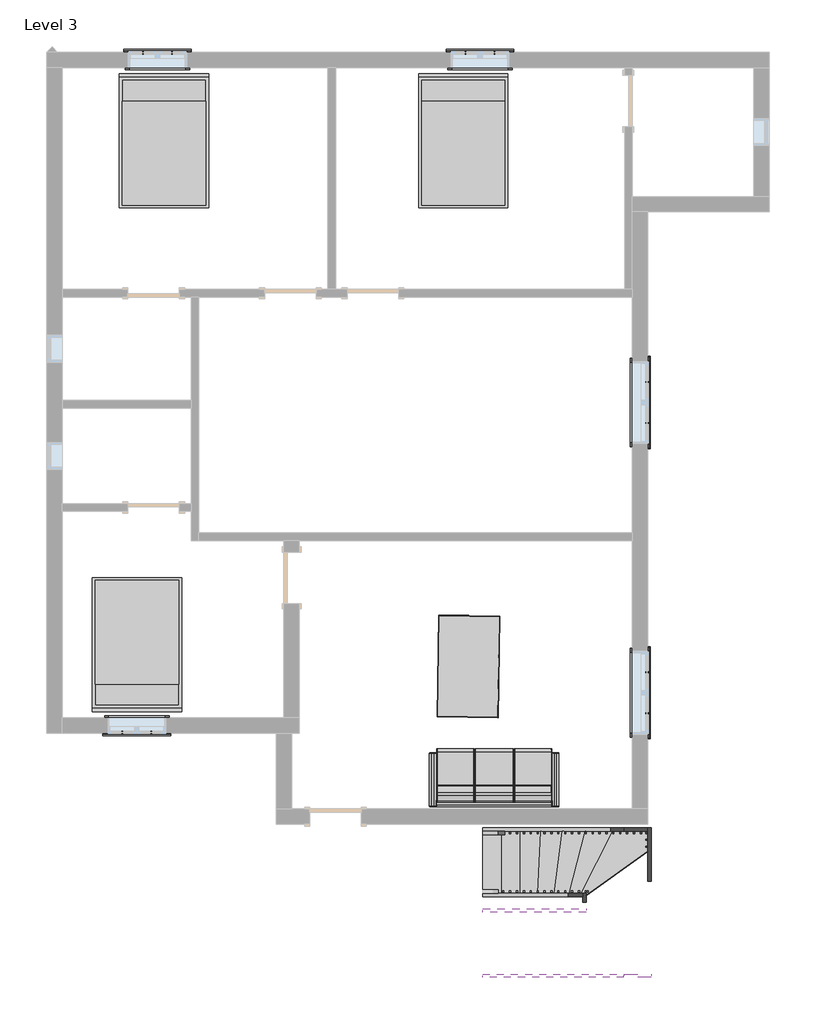
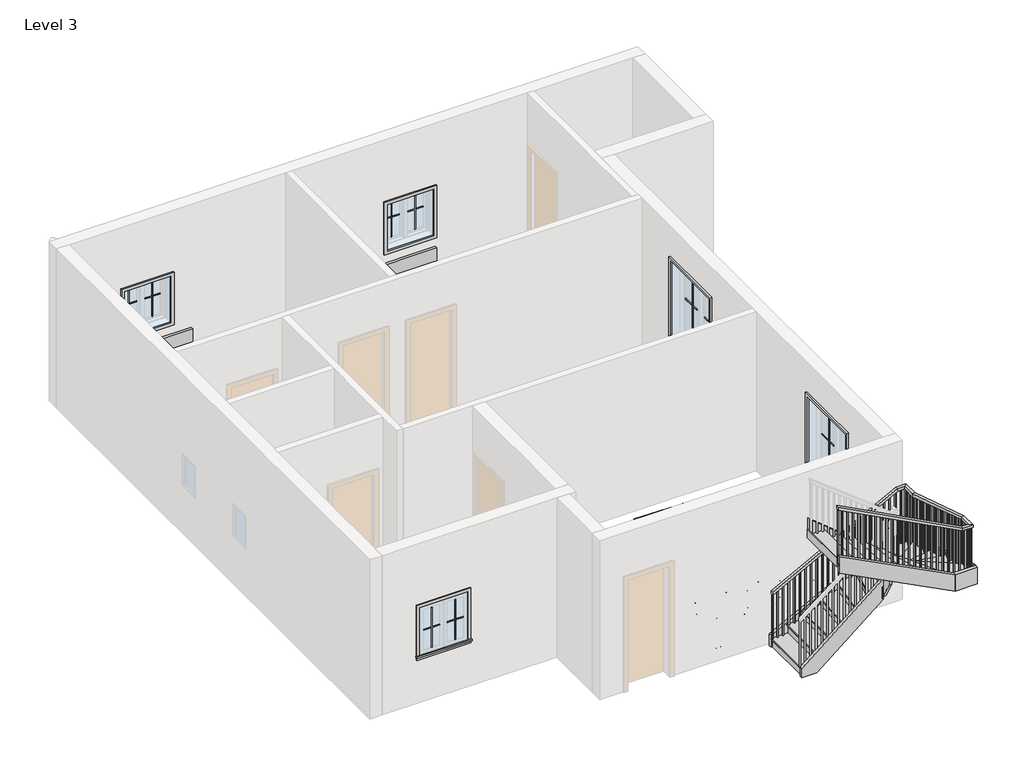
# One storey, part 2 of 2: 20 proxies, 8 members, 5 furniture elements, 1 railing, 1 stair flight.
"""IFC4 building model written with IfcOpenShell, lengths in millimetres."""

from ifc_helpers import new_model, si_unit, frame, origin, place, context, project, spatial, polyline, outline, extrude, faceted_brep, transform, mapped, element, save
from components import muntin_pattern_2x2_muntin_pattern_2x2_b3fe6957, muntin_pattern_2x2_muntin_pattern_2x2_3e0ecaf2, muntin_pattern_2x2_muntin_pattern_2x2_6dad3731, muntin_pattern_2x2_muntin_pattern_2x2_a30a3345, trim_window_exterior_flat_with_sill_41619996, trim_window_exterior_flat_with_sill_92b9b949, trim_window_interior_flat_picture_frame_51c85655, trim_window_interior_flat_picture_frame_3bb882cf, furniture_2fc85b74, furniture_29a9adb8, furniture_57072a26, bed_17739_bed_17739_15c61121, dining_table_14755_dining_table_14755_d89cb775, stair_flight_0756a42a

model = new_model("IFC4")

# Units and contexts
model_context = context("Model", 3, world=origin())
ifc_project = project(units=[si_unit("LENGTHUNIT", "METRE", prefix="MILLI")], contexts=[model_context])

# Site, building, storey
site = spatial("IfcSite", under=ifc_project)
building = spatial("IfcBuilding", under=site)
storey = spatial("IfcBuildingStorey", under=building, Name="Level 3", Elevation=3200.4)

# Proxies
placement = place(None, origin())
muntin_pattern_2x2_muntin_pattern_2x2_shape = muntin_pattern_2x2_muntin_pattern_2x2_b3fe6957(model_context)
element("IfcBuildingElementProxy", 1, Name="Muntin Pattern_2x2 : Muntin Pattern_2x2", ObjectType="Muntin Pattern_2x2 : Muntin Pattern_2x2", at=placement, inside=storey, context=model_context, shape_type="MappedRepresentation", body=[
    mapped(muntin_pattern_2x2_muntin_pattern_2x2_shape, transform((-4708.0540084, 8034.3685985, 4184.65), x_axis=(1.0, 0.0, 0.0), y_axis=(0.0, 1.0, 0.0), z_axis=(0.0, 0.0, 1.0))),
])
element("IfcBuildingElementProxy", 2, Name="Muntin Pattern_2x2 : Muntin Pattern_2x2", ObjectType="Muntin Pattern_2x2 : Muntin Pattern_2x2", at=placement, inside=storey, context=model_context, shape_type="MappedRepresentation", body=[
    mapped(muntin_pattern_2x2_muntin_pattern_2x2_shape, transform((54.4459916, 8034.3685985, 4184.65), x_axis=(1.0, 0.0, 0.0), y_axis=(0.0, 1.0, 0.0), z_axis=(0.0, 0.0, 1.0))),
])
element("IfcBuildingElementProxy", 3, Name="Muntin Pattern_2x2 : Muntin Pattern_2x2", ObjectType="Muntin Pattern_2x2 : Muntin Pattern_2x2", at=placement, inside=storey, context=model_context, shape_type="MappedRepresentation", body=[
    mapped(muntin_pattern_2x2_muntin_pattern_2x2_shape, transform((-4584.2290084, -2004.9814015, 4184.65), x_axis=(-1.0, 0.0, 0.0), y_axis=(0.0, -1.0, 0.0), z_axis=(0.0, 0.0, 1.0))),
])
muntin_pattern_2x2_muntin_pattern_2x2_2_shape = muntin_pattern_2x2_muntin_pattern_2x2_3e0ecaf2(model_context)
element("IfcBuildingElementProxy", 4, Name="Muntin Pattern_2x2 : Muntin Pattern_2x2", ObjectType="Muntin Pattern_2x2 : Muntin Pattern_2x2", at=placement, inside=storey, context=model_context, shape_type="MappedRepresentation", body=[
    mapped(muntin_pattern_2x2_muntin_pattern_2x2_2_shape, transform((-4279.4290084, 8034.3685985, 4184.65), x_axis=(-1.0, 0.0, 0.0), y_axis=(0.0, -1.0, 0.0), z_axis=(0.0, 0.0, 1.0))),
])
element("IfcBuildingElementProxy", 5, Name="Muntin Pattern_2x2 : Muntin Pattern_2x2", ObjectType="Muntin Pattern_2x2 : Muntin Pattern_2x2", at=placement, inside=storey, context=model_context, shape_type="MappedRepresentation", body=[
    mapped(muntin_pattern_2x2_muntin_pattern_2x2_2_shape, transform((483.0709916, 8034.3685985, 4184.65), x_axis=(-1.0, 0.0, 0.0), y_axis=(0.0, -1.0, 0.0), z_axis=(0.0, 0.0, 1.0))),
])
element("IfcBuildingElementProxy", 6, Name="Muntin Pattern_2x2 : Muntin Pattern_2x2", ObjectType="Muntin Pattern_2x2 : Muntin Pattern_2x2", at=placement, inside=storey, context=model_context, shape_type="MappedRepresentation", body=[
    mapped(muntin_pattern_2x2_muntin_pattern_2x2_2_shape, transform((-5012.8540084, -2004.9814015, 4184.65), x_axis=(1.0, 0.0, 0.0), y_axis=(0.0, 1.0, 0.0), z_axis=(0.0, 0.0, 1.0))),
])
muntin_pattern_2x2_muntin_pattern_2x2_3_shape = muntin_pattern_2x2_muntin_pattern_2x2_6dad3731(model_context)
element("IfcBuildingElementProxy", 7, Name="Muntin Pattern_2x2 : Muntin Pattern_2x2", ObjectType="Muntin Pattern_2x2 : Muntin Pattern_2x2", at=placement, inside=storey, context=model_context, shape_type="MappedRepresentation", body=[
    mapped(muntin_pattern_2x2_muntin_pattern_2x2_3_shape, transform((2735.7334916, -1114.3939015, 4184.65), x_axis=(0.0, -1.0, 0.0), y_axis=(1.0, 0.0, 0.0), z_axis=(0.0, 0.0, 1.0))),
])
element("IfcBuildingElementProxy", 8, Name="Muntin Pattern_2x2 : Muntin Pattern_2x2", ObjectType="Muntin Pattern_2x2 : Muntin Pattern_2x2", at=placement, inside=storey, context=model_context, shape_type="MappedRepresentation", body=[
    mapped(muntin_pattern_2x2_muntin_pattern_2x2_3_shape, transform((2735.7334916, 3171.8560985, 4184.65), x_axis=(0.0, -1.0, 0.0), y_axis=(1.0, 0.0, 0.0), z_axis=(0.0, 0.0, 1.0))),
])
muntin_pattern_2x2_muntin_pattern_2x2_4_shape = muntin_pattern_2x2_muntin_pattern_2x2_a30a3345(model_context)
element("IfcBuildingElementProxy", 9, Name="Muntin Pattern_2x2 : Muntin Pattern_2x2", ObjectType="Muntin Pattern_2x2 : Muntin Pattern_2x2", at=placement, inside=storey, context=model_context, shape_type="MappedRepresentation", body=[
    mapped(muntin_pattern_2x2_muntin_pattern_2x2_4_shape, transform((2735.7334916, -1720.8189015, 4184.65), x_axis=(0.0, 1.0, 0.0), y_axis=(-1.0, 0.0, 0.0), z_axis=(0.0, 0.0, 1.0))),
])
element("IfcBuildingElementProxy", 10, Name="Muntin Pattern_2x2 : Muntin Pattern_2x2", ObjectType="Muntin Pattern_2x2 : Muntin Pattern_2x2", at=placement, inside=storey, context=model_context, shape_type="MappedRepresentation", body=[
    mapped(muntin_pattern_2x2_muntin_pattern_2x2_4_shape, transform((2735.7334916, 2565.4310985, 4184.65), x_axis=(0.0, 1.0, 0.0), y_axis=(-1.0, 0.0, 0.0), z_axis=(0.0, 0.0, 1.0))),
])
trim_window_exterior_flat_with_sill_shape = trim_window_exterior_flat_with_sill_41619996(model_context)
element("IfcBuildingElementProxy", 11, Name="Trim-Window-Exterior-Flat : with Sill", ObjectType="Trim-Window-Exterior-Flat : with Sill", at=placement, inside=storey, context=model_context, shape_type="MappedRepresentation", body=[
    mapped(trim_window_exterior_flat_with_sill_shape, transform((-4493.7415084, 8043.8935985, 5029.2), x_axis=(-1.0, 0.0, 0.0), y_axis=(0.0, 0.0, 1.0), z_axis=(0.0, 1.0, 0.0))),
])
element("IfcBuildingElementProxy", 12, Name="Trim-Window-Exterior-Flat : with Sill", ObjectType="Trim-Window-Exterior-Flat : with Sill", at=placement, inside=storey, context=model_context, shape_type="MappedRepresentation", body=[
    mapped(trim_window_exterior_flat_with_sill_shape, transform((268.7584916, 8043.8935985, 5029.2), x_axis=(-1.0, 0.0, 0.0), y_axis=(0.0, 0.0, 1.0), z_axis=(0.0, 1.0, 0.0))),
])
element("IfcBuildingElementProxy", 13, Name="Trim-Window-Exterior-Flat : with Sill", ObjectType="Trim-Window-Exterior-Flat : with Sill", at=placement, inside=storey, context=model_context, shape_type="MappedRepresentation", body=[
    mapped(trim_window_exterior_flat_with_sill_shape, transform((-4798.5415084, -2014.5064015, 5029.2), x_axis=(1.0, 0.0, 0.0), y_axis=(0.0, 0.0, 1.0), z_axis=(0.0, -1.0, 0.0))),
])
trim_window_exterior_flat_with_sill_2_shape = trim_window_exterior_flat_with_sill_92b9b949(model_context)
element("IfcBuildingElementProxy", 14, Name="Trim-Window-Exterior-Flat : with Sill", ObjectType="Trim-Window-Exterior-Flat : with Sill", at=placement, inside=storey, context=model_context, shape_type="MappedRepresentation", body=[
    mapped(trim_window_exterior_flat_with_sill_2_shape, transform((2745.2584916, -1417.6064015, 5638.8), x_axis=(0.0, 1.0, 0.0), y_axis=(0.0, 0.0, 1.0), z_axis=(1.0, 0.0, 0.0))),
])
element("IfcBuildingElementProxy", 15, Name="Trim-Window-Exterior-Flat : with Sill", ObjectType="Trim-Window-Exterior-Flat : with Sill", at=placement, inside=storey, context=model_context, shape_type="MappedRepresentation", body=[
    mapped(trim_window_exterior_flat_with_sill_2_shape, transform((2745.2584916, 2868.6435985, 5638.8), x_axis=(0.0, 1.0, 0.0), y_axis=(0.0, 0.0, 1.0), z_axis=(1.0, 0.0, 0.0))),
])
trim_window_interior_flat_picture_frame_shape = trim_window_interior_flat_picture_frame_51c85655(model_context)
element("IfcBuildingElementProxy", 16, Name="Trim-Window-Interior-Flat : Picture Frame", ObjectType="Trim-Window-Interior-Flat : Picture Frame", at=placement, inside=storey, context=model_context, shape_type="MappedRepresentation", body=[
    mapped(trim_window_interior_flat_picture_frame_shape, transform((-4493.7415084, 7815.2935985, 5029.2), x_axis=(1.0, 0.0, 0.0), y_axis=(0.0, 0.0, 1.0), z_axis=(0.0, -1.0, 0.0))),
])
element("IfcBuildingElementProxy", 17, Name="Trim-Window-Interior-Flat : Picture Frame", ObjectType="Trim-Window-Interior-Flat : Picture Frame", at=placement, inside=storey, context=model_context, shape_type="MappedRepresentation", body=[
    mapped(trim_window_interior_flat_picture_frame_shape, transform((268.7584916, 7815.2935985, 5029.2), x_axis=(1.0, 0.0, 0.0), y_axis=(0.0, 0.0, 1.0), z_axis=(0.0, -1.0, 0.0))),
])
element("IfcBuildingElementProxy", 18, Name="Trim-Window-Interior-Flat : Picture Frame", ObjectType="Trim-Window-Interior-Flat : Picture Frame", at=placement, inside=storey, context=model_context, shape_type="MappedRepresentation", body=[
    mapped(trim_window_interior_flat_picture_frame_shape, transform((-4798.5415084, -1785.9064015, 5029.2), x_axis=(-1.0, 0.0, 0.0), y_axis=(0.0, 0.0, 1.0), z_axis=(0.0, 1.0, 0.0))),
])
trim_window_interior_flat_picture_frame_2_shape = trim_window_interior_flat_picture_frame_3bb882cf(model_context)
element("IfcBuildingElementProxy", 19, Name="Trim-Window-Interior-Flat : Picture Frame", ObjectType="Trim-Window-Interior-Flat : Picture Frame", at=placement, inside=storey, context=model_context, shape_type="MappedRepresentation", body=[
    mapped(trim_window_interior_flat_picture_frame_2_shape, transform((2516.6584916, -1417.6064015, 5638.8), x_axis=(0.0, -1.0, 0.0), y_axis=(0.0, 0.0, 1.0), z_axis=(-1.0, 0.0, 0.0))),
])
element("IfcBuildingElementProxy", 20, Name="Trim-Window-Interior-Flat : Picture Frame", ObjectType="Trim-Window-Interior-Flat : Picture Frame", at=placement, inside=storey, context=model_context, shape_type="MappedRepresentation", body=[
    mapped(trim_window_interior_flat_picture_frame_2_shape, transform((2516.6584916, 2868.6435985, 5638.8), x_axis=(0.0, -1.0, 0.0), y_axis=(0.0, 0.0, 1.0), z_axis=(-1.0, 0.0, 0.0))),
])

# Furniture
furniture_shape = furniture_2fc85b74(model_context)
furniture_2_shape = furniture_29a9adb8(model_context)
furniture_3_shape = furniture_57072a26(model_context)
element("IfcFurniture", 21, at=placement, inside=storey, context=model_context, shape_type="MappedRepresentation", body=[
    mapped(furniture_shape, transform((477.9947981, -2301.7922014, 3200.4), x_axis=(-1.0, 0.0, 0.0), y_axis=(0.0, -1.0, 0.0), z_axis=(0.0, 0.0, 1.0))),
    mapped(furniture_2_shape, transform((477.9947981, -2301.7922014, 3200.4), x_axis=(-1.0, 0.0, 0.0), y_axis=(0.0, -1.0, 0.0), z_axis=(0.0, 0.0, 1.0))),
    mapped(furniture_3_shape, transform((477.9947981, -2301.7922014, 3200.4), x_axis=(-1.0, 0.0, 0.0), y_axis=(0.0, -1.0, 0.0), z_axis=(0.0, 0.0, 1.0))),
])
bed_17739_bed_17739_shape = bed_17739_bed_17739_15c61121(model_context)
element("IfcFurniture", 22, ObjectType="Bed_17739 : Bed_17739", at=placement, inside=storey, context=model_context, shape_type="MappedRepresentation", body=[
    mapped(bed_17739_bed_17739_shape, transform((-4398.4915084, 6710.3935985, 3200.4), x_axis=(1.0, 0.0, 0.0), y_axis=(0.0, 1.0, 0.0), z_axis=(0.0, 0.0, 1.0))),
])
element("IfcFurniture", 23, ObjectType="Bed_17739 : Bed_17739", at=placement, inside=storey, context=model_context, shape_type="MappedRepresentation", body=[
    mapped(bed_17739_bed_17739_shape, transform((21.1084916, 6710.3935985, 3200.4), x_axis=(1.0, 0.0, 0.0), y_axis=(0.0, 1.0, 0.0), z_axis=(0.0, 0.0, 1.0))),
])
element("IfcFurniture", 24, ObjectType="Bed_17739 : Bed_17739", at=placement, inside=storey, context=model_context, shape_type="MappedRepresentation", body=[
    mapped(bed_17739_bed_17739_shape, transform((-4798.5415084, -681.0064015, 3200.4), x_axis=(-1.0, 0.0, 0.0), y_axis=(0.0, -1.0, 0.0), z_axis=(0.0, 0.0, 1.0))),
])
dining_table_14755_dining_table_14755_shape = dining_table_14755_dining_table_14755_d89cb775(model_context)
element("IfcFurniture", 25, ObjectType="Dining_table_14755 : Dining_table_14755", at=placement, inside=storey, context=model_context, shape_type="MappedRepresentation", body=[
    mapped(dining_table_14755_dining_table_14755_shape, transform((535.647979, -1785.9064015, 3200.4), x_axis=(0.016088397262737867, 0.9998705733611308, 0.0), y_axis=(-0.9998705733611308, 0.016088397262737867, 0.0), z_axis=(0.0, 0.0, 1.0))),
])

# Members
element("IfcMember", 26, ObjectType="Stringer - 2\" Width", at=placement, inside=storey, context=model_context, shape_type="SweptSolid", body=[
    extrude(outline(polyline([(3430.039954, 306.9570026), (3200.4, 306.9570026), (3200.4, 526.7193201), (4162.900629, 2394.3741942), (4505.7956453, 2394.3741942), (3430.039954, 306.9570026)])), frame((0.0, -3462.3064015, 0.0), z_axis=(0.0, 1.0, 0.0), x_axis=(0.0, 0.0, 1.0)), (0.0, 0.0, 1.0), 50.8),
])
element("IfcMember", 27, ObjectType="Stringer - 2\" Width", at=placement, inside=storey, context=model_context, shape_type="SweptSolid", body=[
    extrude(outline(polyline([(2394.3741942, -3462.3064015), (2394.3741942, -3411.5064015), (2749.0886944, -3411.5064015), (2749.0886944, -3462.3064015), (2394.3741942, -3462.3064015)])), frame((0.0, 0.0, 4162.900629), z_axis=(0.0, 0.0, 1.0), x_axis=(1.0, 0.0, 0.0)), (0.0, 0.0, 1.0), 342.8950162),
])
element("IfcMember", 28, ObjectType="Stringer - 2\" Width", at=placement, inside=storey, context=model_context, shape_type="SweptSolid", body=[
    extrude(outline(polyline([(-3411.5064015, 4489.4952212), (-3411.5064015, 4200.9956453), (-3581.0288845, 4200.9956453), (-5570.5064015, 4839.3682298), (-5570.5064015, 5170.3972697), (-5533.5262842, 5170.3972697), (-3411.5064015, 4489.4952212)])), frame((2749.0886944, 0.0, 0.0), z_axis=(1.0, 0.0, 0.0), x_axis=(0.0, 1.0, 0.0)), (0.0, 0.0, 1.0), 50.8),
])
element("IfcMember", 29, ObjectType="Stringer - 2\" Width", at=placement, inside=storey, context=model_context, shape_type="SweptSolid", body=[
    extrude(outline(polyline([(2799.8886944, -5570.5064015), (2799.8886944, -5621.3064015), (2394.3741942, -5621.3064015), (2394.3741942, -5570.5064015), (2799.8886944, -5570.5064015)])), frame((0.0, 0.0, 4850.2904473), z_axis=(0.0, 0.0, 1.0), x_axis=(1.0, 0.0, 0.0)), (0.0, 0.0, 1.0), 320.1068224),
])
element("IfcMember", 30, ObjectType="Stringer - 2\" Width", at=placement, inside=storey, context=model_context, shape_type="SweptSolid", body=[
    extrude(outline(polyline([(4850.2904473, 2394.3741942), (5170.3972697, 2394.3741942), (6246.1529609, 306.9570026), (5926.0461385, 306.9570026), (4850.2904473, 2394.3741942)])), frame((0.0, -5621.3064015, 0.0), z_axis=(0.0, 1.0, 0.0), x_axis=(0.0, 0.0, 1.0)), (0.0, 0.0, 1.0), 50.8),
])
element("IfcMember", 31, ObjectType="Stringer - 2\" Width", at=placement, inside=storey, context=model_context, shape_type="SweptSolid", body=[
    extrude(outline(polyline([(3376.5764461, 306.9570026), (3200.4, 306.9570026), (3200.4, 573.2186471), (4187.5410923, 1783.8886944), (4580.818648, 1783.8886944), (3376.5764461, 306.9570026)])), frame((0.0, -4427.5064015, 0.0), z_axis=(0.0, 1.0, 0.0), x_axis=(0.0, 0.0, 1.0)), (0.0, 0.0, 1.0), 50.8),
])
element("IfcMember", 32, ObjectType="Stringer - 2\" Width", at=placement, inside=storey, context=model_context, shape_type="SweptSolid", body=[
    extrude(outline(polyline([(-4376.7064015, 4773.6682978), (-4376.7064015, 4228.9617647), (-4410.9486188, 4228.9617647), (-4605.3064015, 4560.865107), (-4605.3064015, 5126.5409689), (-4583.3435189, 5126.5409689), (-4376.7064015, 4773.6682978)])), frame((1783.8886944, 0.0, 0.0), z_axis=(1.0, 0.0, 0.0), x_axis=(0.0, 1.0, 0.0)), (0.0, 0.0, 1.0), 50.8),
])
element("IfcMember", 33, ObjectType="Stringer - 2\" Width", at=placement, inside=storey, context=model_context, shape_type="SweptSolid", body=[
    extrude(outline(polyline([(4733.2634131, 1834.6886944), (5126.5409689, 1834.6886944), (6372.2038432, 306.9570026), (5978.9262875, 306.9570026), (4733.2634131, 1834.6886944)])), frame((0.0, -4656.1064015, 0.0), z_axis=(0.0, 1.0, 0.0), x_axis=(0.0, 0.0, 1.0)), (0.0, 0.0, 1.0), 50.8),
])

# Railing
element("IfcRailing", 34, ObjectType="Handrail - Rectangular", at=placement, inside=storey, context=model_context, shape_type="SolidModel", body=[
    faceted_brep([(306.9570026, -3462.3064015, 4284.1333333), (306.9570026, -3462.3064015, 4226.6742652), (306.9570026, -3513.1064015, 4226.6742652), (306.9570026, -3513.1064015, 4284.1333333), (2564.6820646, -3462.3064015, 5477.4239201), (2577.2811291, -3462.3064015, 5426.6239201), (2577.2811291, -3513.1064015, 5426.6239201), (2564.6820646, -3513.1064015, 5477.4239201), (2749.0886944, -3462.3064015, 5477.4239201), (2749.0886944, -3462.3064015, 5426.6239201), (2698.2886944, -3513.1064015, 5426.6239201), (2698.2886944, -3513.1064015, 5477.4239201), (2749.0886944, -3749.6182836, 5477.4239201), (2749.0886944, -3757.5688598, 5426.6239201), (2698.2886944, -3757.5688598, 5426.6239201), (2698.2886944, -3749.6182836, 5477.4239201), (2749.0886944, -5283.1945194, 5969.5094132), (2749.0886944, -5291.1450955, 5918.7094132), (2698.2886944, -5291.1450955, 5918.7094132), (2698.2886944, -5283.1945194, 5969.5094132), (2749.0886944, -5570.5064015, 5969.5094132), (2749.0886944, -5570.5064015, 5918.7094132), (2698.2886944, -5519.7064015, 5918.7094132), (2698.2886944, -5519.7064015, 5969.5094132), (2564.6820646, -5570.5064015, 5969.5094132), (2552.0830001, -5570.5064015, 5918.7094132), (2552.0830001, -5519.7064015, 5918.7094132), (2564.6820646, -5519.7064015, 5969.5094132), (306.9570026, -5570.5064015, 7162.8), (306.9570026, -5519.7064015, 7162.8), (306.9570026, -5519.7064015, 7105.3409318), (306.9570026, -5570.5064015, 7105.3409318)], [[[0, 1, 2, 3]], [[1, 0, 4, 5]], [[2, 1, 5, 6]], [[3, 2, 6, 7]], [[0, 3, 7, 4]], [[5, 4, 8, 9]], [[6, 5, 9, 10]], [[7, 6, 10, 11]], [[4, 7, 11, 8]], [[9, 8, 12, 13]], [[10, 9, 13, 14]], [[11, 10, 14, 15]], [[8, 11, 15, 12]], [[13, 12, 16, 17]], [[14, 13, 17, 18]], [[15, 14, 18, 19]], [[12, 15, 19, 16]], [[17, 16, 20, 21]], [[18, 17, 21, 22]], [[19, 18, 22, 23]], [[16, 19, 23, 20]], [[21, 20, 24, 25]], [[22, 21, 25, 26]], [[23, 22, 26, 27]], [[20, 23, 27, 24]], [[28, 29, 30, 31]], [[25, 24, 28, 31]], [[26, 25, 31, 30]], [[27, 26, 30, 29]], [[24, 27, 29, 28]]]),
    extrude(outline(polyline([(7068.1284102, 377.3636944), (6079.0666667, 377.3636944), (6079.0666667, 396.4136944), (7058.0597858, 396.4136944), (7068.1284102, 377.3636944)])), frame((0.0, -5554.6314015, 0.0), z_axis=(0.0, 1.0, 0.0), x_axis=(0.0, 0.0, 1.0)), (0.0, 0.0, 1.0), 19.05),
    extrude(outline(polyline([(7014.42908, 478.9636944), (6079.0666667, 478.9636944), (6079.0666667, 498.0136944), (7004.3604556, 498.0136944), (7014.42908, 478.9636944)])), frame((0.0, -5554.6314015, 0.0), z_axis=(0.0, 1.0, 0.0), x_axis=(0.0, 0.0, 1.0)), (0.0, 0.0, 1.0), 19.05),
    extrude(outline(polyline([(6960.7297498, 580.5636944), (5909.7333333, 580.5636944), (5909.7333333, 599.6136944), (6950.6611254, 599.6136944), (6960.7297498, 580.5636944)])), frame((0.0, -5554.6314015, 0.0), z_axis=(0.0, 1.0, 0.0), x_axis=(0.0, 0.0, 1.0)), (0.0, 0.0, 1.0), 19.05),
    extrude(outline(polyline([(6907.0304196, 682.1636944), (5909.7333333, 682.1636944), (5909.7333333, 701.2136944), (6896.9617952, 701.2136944), (6907.0304196, 682.1636944)])), frame((0.0, -5554.6314015, 0.0), z_axis=(0.0, 1.0, 0.0), x_axis=(0.0, 0.0, 1.0)), (0.0, 0.0, 1.0), 19.05),
    extrude(outline(polyline([(6853.3310894, 783.7636944), (5909.7333333, 783.7636944), (5909.7333333, 802.8136944), (6843.262465, 802.8136944), (6853.3310894, 783.7636944)])), frame((0.0, -5554.6314015, 0.0), z_axis=(0.0, 1.0, 0.0), x_axis=(0.0, 0.0, 1.0)), (0.0, 0.0, 1.0), 19.05),
    extrude(outline(polyline([(6799.6317592, 885.3636944), (5740.4, 885.3636944), (5740.4, 904.4136944), (6789.5631348, 904.4136944), (6799.6317592, 885.3636944)])), frame((0.0, -5554.6314015, 0.0), z_axis=(0.0, 1.0, 0.0), x_axis=(0.0, 0.0, 1.0)), (0.0, 0.0, 1.0), 19.05),
    extrude(outline(polyline([(6745.932429, 986.9636944), (5740.4, 986.9636944), (5740.4, 1006.0136944), (6735.8638046, 1006.0136944), (6745.932429, 986.9636944)])), frame((0.0, -5554.6314015, 0.0), z_axis=(0.0, 1.0, 0.0), x_axis=(0.0, 0.0, 1.0)), (0.0, 0.0, 1.0), 19.05),
    extrude(outline(polyline([(6692.2330988, 1088.5636944), (5740.4, 1088.5636944), (5740.4, 1107.6136944), (6682.1644744, 1107.6136944), (6692.2330988, 1088.5636944)])), frame((0.0, -5554.6314015, 0.0), z_axis=(0.0, 1.0, 0.0), x_axis=(0.0, 0.0, 1.0)), (0.0, 0.0, 1.0), 19.05),
    extrude(outline(polyline([(6638.5337686, 1190.1636944), (5571.0666667, 1190.1636944), (5571.0666667, 1209.2136944), (6628.4651442, 1209.2136944), (6638.5337686, 1190.1636944)])), frame((0.0, -5554.6314015, 0.0), z_axis=(0.0, 1.0, 0.0), x_axis=(0.0, 0.0, 1.0)), (0.0, 0.0, 1.0), 19.05),
    extrude(outline(polyline([(6584.8344384, 1291.7636944), (5571.0666667, 1291.7636944), (5571.0666667, 1310.8136944), (6574.765814, 1310.8136944), (6584.8344384, 1291.7636944)])), frame((0.0, -5554.6314015, 0.0), z_axis=(0.0, 1.0, 0.0), x_axis=(0.0, 0.0, 1.0)), (0.0, 0.0, 1.0), 19.05),
    extrude(outline(polyline([(6531.1351082, 1393.3636944), (5571.0666667, 1393.3636944), (5571.0666667, 1412.4136944), (6521.0664838, 1412.4136944), (6531.1351082, 1393.3636944)])), frame((0.0, -5554.6314015, 0.0), z_axis=(0.0, 1.0, 0.0), x_axis=(0.0, 0.0, 1.0)), (0.0, 0.0, 1.0), 19.05),
    extrude(outline(polyline([(6477.435778, 1494.9636944), (5401.7333333, 1494.9636944), (5401.7333333, 1514.0136944), (6467.3671536, 1514.0136944), (6477.435778, 1494.9636944)])), frame((0.0, -5554.6314015, 0.0), z_axis=(0.0, 1.0, 0.0), x_axis=(0.0, 0.0, 1.0)), (0.0, 0.0, 1.0), 19.05),
    extrude(outline(polyline([(6423.7364478, 1596.5636944), (5401.7333333, 1596.5636944), (5401.7333333, 1615.6136944), (6413.6678234, 1615.6136944), (6423.7364478, 1596.5636944)])), frame((0.0, -5554.6314015, 0.0), z_axis=(0.0, 1.0, 0.0), x_axis=(0.0, 0.0, 1.0)), (0.0, 0.0, 1.0), 19.05),
    extrude(outline(polyline([(6370.0371176, 1698.1636944), (5401.7333333, 1698.1636944), (5401.7333333, 1717.2136944), (6359.9684932, 1717.2136944), (6370.0371176, 1698.1636944)])), frame((0.0, -5554.6314015, 0.0), z_axis=(0.0, 1.0, 0.0), x_axis=(0.0, 0.0, 1.0)), (0.0, 0.0, 1.0), 19.05),
    extrude(outline(polyline([(6316.3377874, 1799.7636944), (5401.7333333, 1799.7636944), (5401.7333333, 1818.8136944), (6306.269163, 1818.8136944), (6316.3377874, 1799.7636944)])), frame((0.0, -5554.6314015, 0.0), z_axis=(0.0, 1.0, 0.0), x_axis=(0.0, 0.0, 1.0)), (0.0, 0.0, 1.0), 19.05),
    extrude(outline(polyline([(6262.6384572, 1901.3636944), (5232.4, 1901.3636944), (5232.4, 1920.4136944), (6252.5698328, 1920.4136944), (6262.6384572, 1901.3636944)])), frame((0.0, -5554.6314015, 0.0), z_axis=(0.0, 1.0, 0.0), x_axis=(0.0, 0.0, 1.0)), (0.0, 0.0, 1.0), 19.05),
    extrude(outline(polyline([(6208.939127, 2002.9636944), (5232.4, 2002.9636944), (5232.4, 2022.0136944), (6198.8705026, 2022.0136944), (6208.939127, 2002.9636944)])), frame((0.0, -5554.6314015, 0.0), z_axis=(0.0, 1.0, 0.0), x_axis=(0.0, 0.0, 1.0)), (0.0, 0.0, 1.0), 19.05),
    extrude(outline(polyline([(6155.2397968, 2104.5636944), (5232.4, 2104.5636944), (5232.4, 2123.6136944), (6145.1711724, 2123.6136944), (6155.2397968, 2104.5636944)])), frame((0.0, -5554.6314015, 0.0), z_axis=(0.0, 1.0, 0.0), x_axis=(0.0, 0.0, 1.0)), (0.0, 0.0, 1.0), 19.05),
    extrude(outline(polyline([(6101.5404666, 2206.1636944), (5232.4, 2206.1636944), (5232.4, 2225.2136944), (6091.4718422, 2225.2136944), (6101.5404666, 2206.1636944)])), frame((0.0, -5554.6314015, 0.0), z_axis=(0.0, 1.0, 0.0), x_axis=(0.0, 0.0, 1.0)), (0.0, 0.0, 1.0), 19.05),
    extrude(outline(polyline([(6047.8411364, 2307.7636944), (5063.0666667, 2307.7636944), (5063.0666667, 2326.8136944), (6037.772512, 2326.8136944), (6047.8411364, 2307.7636944)])), frame((0.0, -5554.6314015, 0.0), z_axis=(0.0, 1.0, 0.0), x_axis=(0.0, 0.0, 1.0)), (0.0, 0.0, 1.0), 19.05),
    extrude(outline(polyline([(5994.1418062, 2409.3636944), (5063.0666667, 2409.3636944), (5063.0666667, 2428.4136944), (5984.0731818, 2428.4136944), (5994.1418062, 2409.3636944)])), frame((0.0, -5554.6314015, 0.0), z_axis=(0.0, 1.0, 0.0), x_axis=(0.0, 0.0, 1.0)), (0.0, 0.0, 1.0), 19.05),
    extrude(outline(polyline([(5940.442476, 2510.9636944), (5063.0666667, 2510.9636944), (5063.0666667, 2530.0136944), (5930.3738516, 2530.0136944), (5940.442476, 2510.9636944)])), frame((0.0, -5554.6314015, 0.0), z_axis=(0.0, 1.0, 0.0), x_axis=(0.0, 0.0, 1.0)), (0.0, 0.0, 1.0), 19.05),
    extrude(outline(polyline([(2631.6136944, -5554.6314015), (2612.5636944, -5554.6314015), (2612.5636944, -5535.5814015), (2631.6136944, -5535.5814015), (2631.6136944, -5554.6314015)])), frame((0.0, 0.0, 5063.0666667), z_axis=(0.0, 0.0, 1.0), x_axis=(1.0, 0.0, 0.0)), (0.0, 0.0, 1.0), 855.6427466),
    extrude(outline(polyline([(2733.2136944, -5510.1814015), (2733.2136944, -5529.2314015), (2714.1636944, -5529.2314015), (2714.1636944, -5510.1814015), (2733.2136944, -5510.1814015)])), frame((0.0, 0.0, 5063.0666667), z_axis=(0.0, 0.0, 1.0), x_axis=(1.0, 0.0, 0.0)), (0.0, 0.0, 1.0), 855.6427466),
    extrude(outline(polyline([(2733.2136944, -5408.5814015), (2733.2136944, -5427.6314015), (2714.1636944, -5427.6314015), (2714.1636944, -5408.5814015), (2733.2136944, -5408.5814015)])), frame((0.0, 0.0, 5063.0666667), z_axis=(0.0, 0.0, 1.0), x_axis=(1.0, 0.0, 0.0)), (0.0, 0.0, 1.0), 855.6427466),
    extrude(outline(polyline([(2733.2136944, -5306.9814015), (2733.2136944, -5326.0314015), (2714.1636944, -5326.0314015), (2714.1636944, -5306.9814015), (2733.2136944, -5306.9814015)])), frame((0.0, 0.0, 5063.0666667), z_axis=(0.0, 0.0, 1.0), x_axis=(1.0, 0.0, 0.0)), (0.0, 0.0, 1.0), 855.6427466),
    extrude(outline(polyline([(-5205.3814015, 5891.1900316), (-5205.3814015, 4893.7333333), (-5224.4314015, 4893.7333333), (-5224.4314015, 5897.3026907), (-5205.3814015, 5891.1900316)])), frame((2714.1636944, 0.0, 0.0), z_axis=(1.0, 0.0, 0.0), x_axis=(0.0, 1.0, 0.0)), (0.0, 0.0, 1.0), 19.05),
    extrude(outline(polyline([(-5103.7814015, 5858.5891834), (-5103.7814015, 4893.7333333), (-5122.8314015, 4893.7333333), (-5122.8314015, 5864.7018425), (-5103.7814015, 5858.5891834)])), frame((2714.1636944, 0.0, 0.0), z_axis=(1.0, 0.0, 0.0), x_axis=(0.0, 1.0, 0.0)), (0.0, 0.0, 1.0), 19.05),
    extrude(outline(polyline([(-5002.1814015, 5825.9883352), (-5002.1814015, 4893.7333333), (-5021.2314015, 4893.7333333), (-5021.2314015, 5832.1009942), (-5002.1814015, 5825.9883352)])), frame((2714.1636944, 0.0, 0.0), z_axis=(1.0, 0.0, 0.0), x_axis=(0.0, 1.0, 0.0)), (0.0, 0.0, 1.0), 19.05),
    extrude(outline(polyline([(-4900.5814015, 5793.387487), (-4900.5814015, 4893.7333333), (-4919.6314015, 4893.7333333), (-4919.6314015, 5799.500146), (-4900.5814015, 5793.387487)])), frame((2714.1636944, 0.0, 0.0), z_axis=(1.0, 0.0, 0.0), x_axis=(0.0, 1.0, 0.0)), (0.0, 0.0, 1.0), 19.05),
    extrude(outline(polyline([(-4798.9814015, 5760.7866387), (-4798.9814015, 4893.7333333), (-4818.0314015, 4893.7333333), (-4818.0314015, 5766.8992978), (-4798.9814015, 5760.7866387)])), frame((2714.1636944, 0.0, 0.0), z_axis=(1.0, 0.0, 0.0), x_axis=(0.0, 1.0, 0.0)), (0.0, 0.0, 1.0), 19.05),
    extrude(outline(polyline([(-4697.3814015, 5728.1857905), (-4697.3814015, 4724.4), (-4716.4314015, 4724.4), (-4716.4314015, 5734.2984495), (-4697.3814015, 5728.1857905)])), frame((2714.1636944, 0.0, 0.0), z_axis=(1.0, 0.0, 0.0), x_axis=(0.0, 1.0, 0.0)), (0.0, 0.0, 1.0), 19.05),
    extrude(outline(polyline([(-4595.7814015, 5695.5849423), (-4595.7814015, 4724.4), (-4614.8314015, 4724.4), (-4614.8314015, 5701.6976013), (-4595.7814015, 5695.5849423)])), frame((2714.1636944, 0.0, 0.0), z_axis=(1.0, 0.0, 0.0), x_axis=(0.0, 1.0, 0.0)), (0.0, 0.0, 1.0), 19.05),
    extrude(outline(polyline([(-4494.1814015, 5662.984094), (-4494.1814015, 4724.4), (-4513.2314015, 4724.4), (-4513.2314015, 5669.0967531), (-4494.1814015, 5662.984094)])), frame((2714.1636944, 0.0, 0.0), z_axis=(1.0, 0.0, 0.0), x_axis=(0.0, 1.0, 0.0)), (0.0, 0.0, 1.0), 19.05),
    extrude(outline(polyline([(-4392.5814015, 5630.3832458), (-4392.5814015, 4724.4), (-4411.6314015, 4724.4), (-4411.6314015, 5636.4959049), (-4392.5814015, 5630.3832458)])), frame((2714.1636944, 0.0, 0.0), z_axis=(1.0, 0.0, 0.0), x_axis=(0.0, 1.0, 0.0)), (0.0, 0.0, 1.0), 19.05),
    extrude(outline(polyline([(-4290.9814015, 5597.7823976), (-4290.9814015, 4724.4), (-4310.0314015, 4724.4), (-4310.0314015, 5603.8950566), (-4290.9814015, 5597.7823976)])), frame((2714.1636944, 0.0, 0.0), z_axis=(1.0, 0.0, 0.0), x_axis=(0.0, 1.0, 0.0)), (0.0, 0.0, 1.0), 19.05),
    extrude(outline(polyline([(-4189.3814015, 5565.1815494), (-4189.3814015, 4555.0666667), (-4208.4314015, 4555.0666667), (-4208.4314015, 5571.2942084), (-4189.3814015, 5565.1815494)])), frame((2714.1636944, 0.0, 0.0), z_axis=(1.0, 0.0, 0.0), x_axis=(0.0, 1.0, 0.0)), (0.0, 0.0, 1.0), 19.05),
    extrude(outline(polyline([(-4087.7814015, 5532.5807011), (-4087.7814015, 4555.0666667), (-4106.8314015, 4555.0666667), (-4106.8314015, 5538.6933602), (-4087.7814015, 5532.5807011)])), frame((2714.1636944, 0.0, 0.0), z_axis=(1.0, 0.0, 0.0), x_axis=(0.0, 1.0, 0.0)), (0.0, 0.0, 1.0), 19.05),
    extrude(outline(polyline([(-3986.1814015, 5499.9798529), (-3986.1814015, 4555.0666667), (-4005.2314015, 4555.0666667), (-4005.2314015, 5506.092512), (-3986.1814015, 5499.9798529)])), frame((2714.1636944, 0.0, 0.0), z_axis=(1.0, 0.0, 0.0), x_axis=(0.0, 1.0, 0.0)), (0.0, 0.0, 1.0), 19.05),
    extrude(outline(polyline([(-3884.5814015, 5467.3790047), (-3884.5814015, 4555.0666667), (-3903.6314015, 4555.0666667), (-3903.6314015, 5473.4916637), (-3884.5814015, 5467.3790047)])), frame((2714.1636944, 0.0, 0.0), z_axis=(1.0, 0.0, 0.0), x_axis=(0.0, 1.0, 0.0)), (0.0, 0.0, 1.0), 19.05),
    extrude(outline(polyline([(-3782.9814015, 5434.7781565), (-3782.9814015, 4555.0666667), (-3802.0314015, 4555.0666667), (-3802.0314015, 5440.8908155), (-3782.9814015, 5434.7781565)])), frame((2714.1636944, 0.0, 0.0), z_axis=(1.0, 0.0, 0.0), x_axis=(0.0, 1.0, 0.0)), (0.0, 0.0, 1.0), 19.05),
    extrude(outline(polyline([(2733.2136944, -3681.3814015), (2733.2136944, -3700.4314015), (2714.1636944, -3700.4314015), (2714.1636944, -3681.3814015), (2733.2136944, -3681.3814015)])), frame((0.0, 0.0, 4385.7333333), z_axis=(0.0, 0.0, 1.0), x_axis=(1.0, 0.0, 0.0)), (0.0, 0.0, 1.0), 1040.8905868),
    extrude(outline(polyline([(2733.2136944, -3579.7814015), (2733.2136944, -3598.8314015), (2714.1636944, -3598.8314015), (2714.1636944, -3579.7814015), (2733.2136944, -3579.7814015)])), frame((0.0, 0.0, 4385.7333333), z_axis=(0.0, 0.0, 1.0), x_axis=(1.0, 0.0, 0.0)), (0.0, 0.0, 1.0), 1040.8905868),
    extrude(outline(polyline([(2634.2320026, -3478.1814015), (2653.2820026, -3478.1814015), (2653.2820026, -3497.2314015), (2634.2320026, -3497.2314015), (2634.2320026, -3478.1814015)])), frame((0.0, 0.0, 4385.7333333), z_axis=(0.0, 0.0, 1.0), x_axis=(1.0, 0.0, 0.0)), (0.0, 0.0, 1.0), 1040.8905868),
    extrude(outline(polyline([(5403.0252174, 2532.6320026), (4385.7333333, 2532.6320026), (4385.7333333, 2551.6820026), (5413.0938418, 2551.6820026), (5403.0252174, 2532.6320026)])), frame((0.0, -3497.2314015, 0.0), z_axis=(0.0, 1.0, 0.0), x_axis=(0.0, 0.0, 1.0)), (0.0, 0.0, 1.0), 19.05),
    extrude(outline(polyline([(5349.3258872, 2431.0320026), (4385.7333333, 2431.0320026), (4385.7333333, 2450.0820026), (5359.3945116, 2450.0820026), (5349.3258872, 2431.0320026)])), frame((0.0, -3497.2314015, 0.0), z_axis=(0.0, 1.0, 0.0), x_axis=(0.0, 0.0, 1.0)), (0.0, 0.0, 1.0), 19.05),
    extrude(outline(polyline([(5295.626557, 2329.4320026), (4385.7333333, 2329.4320026), (4385.7333333, 2348.4820026), (5305.6951814, 2348.4820026), (5295.626557, 2329.4320026)])), frame((0.0, -3497.2314015, 0.0), z_axis=(0.0, 1.0, 0.0), x_axis=(0.0, 0.0, 1.0)), (0.0, 0.0, 1.0), 19.05),
    extrude(outline(polyline([(5241.9272268, 2227.8320026), (4385.7333333, 2227.8320026), (4385.7333333, 2246.8820026), (5251.9958512, 2246.8820026), (5241.9272268, 2227.8320026)])), frame((0.0, -3497.2314015, 0.0), z_axis=(0.0, 1.0, 0.0), x_axis=(0.0, 0.0, 1.0)), (0.0, 0.0, 1.0), 19.05),
    extrude(outline(polyline([(5188.2278966, 2126.2320026), (4216.4, 2126.2320026), (4216.4, 2145.2820026), (5198.296521, 2145.2820026), (5188.2278966, 2126.2320026)])), frame((0.0, -3497.2314015, 0.0), z_axis=(0.0, 1.0, 0.0), x_axis=(0.0, 0.0, 1.0)), (0.0, 0.0, 1.0), 19.05),
    extrude(outline(polyline([(5134.5285664, 2024.6320026), (4216.4, 2024.6320026), (4216.4, 2043.6820026), (5144.5971908, 2043.6820026), (5134.5285664, 2024.6320026)])), frame((0.0, -3497.2314015, 0.0), z_axis=(0.0, 1.0, 0.0), x_axis=(0.0, 0.0, 1.0)), (0.0, 0.0, 1.0), 19.05),
    extrude(outline(polyline([(5080.8292362, 1923.0320026), (4216.4, 1923.0320026), (4216.4, 1942.0820026), (5090.8978606, 1942.0820026), (5080.8292362, 1923.0320026)])), frame((0.0, -3497.2314015, 0.0), z_axis=(0.0, 1.0, 0.0), x_axis=(0.0, 0.0, 1.0)), (0.0, 0.0, 1.0), 19.05),
    extrude(outline(polyline([(5027.129906, 1821.4320026), (4216.4, 1821.4320026), (4216.4, 1840.4820026), (5037.1985304, 1840.4820026), (5027.129906, 1821.4320026)])), frame((0.0, -3497.2314015, 0.0), z_axis=(0.0, 1.0, 0.0), x_axis=(0.0, 0.0, 1.0)), (0.0, 0.0, 1.0), 19.05),
    extrude(outline(polyline([(4973.4305758, 1719.8320026), (4047.0666667, 1719.8320026), (4047.0666667, 1738.8820026), (4983.4992002, 1738.8820026), (4973.4305758, 1719.8320026)])), frame((0.0, -3497.2314015, 0.0), z_axis=(0.0, 1.0, 0.0), x_axis=(0.0, 0.0, 1.0)), (0.0, 0.0, 1.0), 19.05),
    extrude(outline(polyline([(4919.7312456, 1618.2320026), (4047.0666667, 1618.2320026), (4047.0666667, 1637.2820026), (4929.79987, 1637.2820026), (4919.7312456, 1618.2320026)])), frame((0.0, -3497.2314015, 0.0), z_axis=(0.0, 1.0, 0.0), x_axis=(0.0, 0.0, 1.0)), (0.0, 0.0, 1.0), 19.05),
    extrude(outline(polyline([(4866.0319154, 1516.6320026), (4047.0666667, 1516.6320026), (4047.0666667, 1535.6820026), (4876.1005398, 1535.6820026), (4866.0319154, 1516.6320026)])), frame((0.0, -3497.2314015, 0.0), z_axis=(0.0, 1.0, 0.0), x_axis=(0.0, 0.0, 1.0)), (0.0, 0.0, 1.0), 19.05),
    extrude(outline(polyline([(4812.3325852, 1415.0320026), (3877.7333333, 1415.0320026), (3877.7333333, 1434.0820026), (4822.4012096, 1434.0820026), (4812.3325852, 1415.0320026)])), frame((0.0, -3497.2314015, 0.0), z_axis=(0.0, 1.0, 0.0), x_axis=(0.0, 0.0, 1.0)), (0.0, 0.0, 1.0), 19.05),
    extrude(outline(polyline([(4758.633255, 1313.4320026), (3877.7333333, 1313.4320026), (3877.7333333, 1332.4820026), (4768.7018794, 1332.4820026), (4758.633255, 1313.4320026)])), frame((0.0, -3497.2314015, 0.0), z_axis=(0.0, 1.0, 0.0), x_axis=(0.0, 0.0, 1.0)), (0.0, 0.0, 1.0), 19.05),
    extrude(outline(polyline([(4704.9339248, 1211.8320026), (3877.7333333, 1211.8320026), (3877.7333333, 1230.8820026), (4715.0025492, 1230.8820026), (4704.9339248, 1211.8320026)])), frame((0.0, -3497.2314015, 0.0), z_axis=(0.0, 1.0, 0.0), x_axis=(0.0, 0.0, 1.0)), (0.0, 0.0, 1.0), 19.05),
    extrude(outline(polyline([(4651.2345946, 1110.2320026), (3708.4, 1110.2320026), (3708.4, 1129.2820026), (4661.303219, 1129.2820026), (4651.2345946, 1110.2320026)])), frame((0.0, -3497.2314015, 0.0), z_axis=(0.0, 1.0, 0.0), x_axis=(0.0, 0.0, 1.0)), (0.0, 0.0, 1.0), 19.05),
    extrude(outline(polyline([(4597.5352644, 1008.6320026), (3708.4, 1008.6320026), (3708.4, 1027.6820026), (4607.6038888, 1027.6820026), (4597.5352644, 1008.6320026)])), frame((0.0, -3497.2314015, 0.0), z_axis=(0.0, 1.0, 0.0), x_axis=(0.0, 0.0, 1.0)), (0.0, 0.0, 1.0), 19.05),
    extrude(outline(polyline([(4543.8359342, 907.0320026), (3708.4, 907.0320026), (3708.4, 926.0820026), (4553.9045586, 926.0820026), (4543.8359342, 907.0320026)])), frame((0.0, -3497.2314015, 0.0), z_axis=(0.0, 1.0, 0.0), x_axis=(0.0, 0.0, 1.0)), (0.0, 0.0, 1.0), 19.05),
    extrude(outline(polyline([(4490.136604, 805.4320026), (3539.0666667, 805.4320026), (3539.0666667, 824.4820026), (4500.2052284, 824.4820026), (4490.136604, 805.4320026)])), frame((0.0, -3497.2314015, 0.0), z_axis=(0.0, 1.0, 0.0), x_axis=(0.0, 0.0, 1.0)), (0.0, 0.0, 1.0), 19.05),
    extrude(outline(polyline([(4436.4372738, 703.8320026), (3539.0666667, 703.8320026), (3539.0666667, 722.8820026), (4446.5058982, 722.8820026), (4436.4372738, 703.8320026)])), frame((0.0, -3497.2314015, 0.0), z_axis=(0.0, 1.0, 0.0), x_axis=(0.0, 0.0, 1.0)), (0.0, 0.0, 1.0), 19.05),
    extrude(outline(polyline([(4382.7379436, 602.2320026), (3539.0666667, 602.2320026), (3539.0666667, 621.2820026), (4392.806568, 621.2820026), (4382.7379436, 602.2320026)])), frame((0.0, -3497.2314015, 0.0), z_axis=(0.0, 1.0, 0.0), x_axis=(0.0, 0.0, 1.0)), (0.0, 0.0, 1.0), 19.05),
    extrude(outline(polyline([(4329.0386134, 500.6320026), (3369.7333333, 500.6320026), (3369.7333333, 519.6820026), (4339.1072378, 519.6820026), (4329.0386134, 500.6320026)])), frame((0.0, -3497.2314015, 0.0), z_axis=(0.0, 1.0, 0.0), x_axis=(0.0, 0.0, 1.0)), (0.0, 0.0, 1.0), 19.05),
    extrude(outline(polyline([(4275.3392831, 399.0320026), (3369.7333333, 399.0320026), (3369.7333333, 418.0820026), (4285.4079076, 418.0820026), (4275.3392831, 399.0320026)])), frame((0.0, -3497.2314015, 0.0), z_axis=(0.0, 1.0, 0.0), x_axis=(0.0, 0.0, 1.0)), (0.0, 0.0, 1.0), 19.05),
    extrude(outline(polyline([(2733.2136944, -5535.5814015), (2733.2136944, -5554.6314015), (2714.1636944, -5554.6314015), (2714.1636944, -5535.5814015), (2733.2136944, -5535.5814015)])), frame((0.0, 0.0, 5063.0666667), z_axis=(0.0, 0.0, 1.0), x_axis=(1.0, 0.0, 0.0)), (0.0, 0.0, 1.0), 855.6427466),
    extrude(outline(polyline([(2714.1636944, -3478.1814015), (2733.2136944, -3478.1814015), (2733.2136944, -3497.2314015), (2714.1636944, -3497.2314015), (2714.1636944, -3478.1814015)])), frame((0.0, 0.0, 4385.7333333), z_axis=(0.0, 0.0, 1.0), x_axis=(1.0, 0.0, 0.0)), (0.0, 0.0, 1.0), 1040.8905868),
    extrude(outline(polyline([(7105.3409318, 306.9570026), (6079.0666667, 306.9570026), (6079.0666667, 326.0070026), (7095.2723074, 326.0070026), (7105.3409318, 306.9570026)])), frame((0.0, -5554.6314015, 0.0), z_axis=(0.0, 1.0, 0.0), x_axis=(0.0, 0.0, 1.0)), (0.0, 0.0, 1.0), 19.05),
    extrude(outline(polyline([(4226.6742652, 306.9570026), (3369.7333333, 306.9570026), (3369.7333333, 326.0070026), (4236.7428896, 326.0070026), (4226.6742652, 306.9570026)])), frame((0.0, -3497.2314015, 0.0), z_axis=(0.0, 1.0, 0.0), x_axis=(0.0, 0.0, 1.0)), (0.0, 0.0, 1.0), 19.05),
])

# Stair flight
stair_flight_shape = stair_flight_0756a42a(model_context)
element("IfcStairFlight", 35, ObjectType="2\" Tread 1\" Nosing 1/4\" Riser", at=placement, inside=storey, context=model_context, shape_type="MappedRepresentation", body=[
    mapped(stair_flight_shape, transform((0.0, 0.0, 0.0), x_axis=(1.0, 0.0, 0.0), y_axis=(0.0, 1.0, 0.0), z_axis=(0.0, 0.0, 1.0))),
])

save(model, "model.ifc")

# Revit data of these elements
# Type "Muntin Pattern_2x2 : Muntin Pattern_2x2"
#   Width [instance default] = 4' - 0"
#   Thickness = 0' - 0 1/2"
#   Height [instance default] = 4' - 0"
#   Distance = 0' - 0 3/4"
#   Interior Material [instance default] = none
#   Exterior Material [instance default] = none
#   Default Elevation = 0
# Type "Trim-Window-Exterior-Flat : with Sill"
#   Trim Width = 0' - 2 1/4"
#   Trim Thickness_Picture Frame = 0' - 1 1/4"
#   Trim Thickness_with Sill = 0' - 0 3/4"
#   Sill Thickness = 0' - 1 1/4"
#   Opening Width [instance default] = 2' - 0"
#   Opening Height [instance default] = 3' - 0"
#   Default Elevation = 4' - 0"
#   Sill = yes
#   Picture Frame = no
#   Trim Material [instance default] = none
# Type "Trim-Window-Interior-Flat : Picture Frame"
#   Trim Thickness_Picture Frame = 0' - 1 1/4"
#   Trim Width = 0' - 2 1/4"
#   Trim Thickness_with Sill = 0' - 0 3/4"
#   Sill Thickness = 0' - 1 1/4"
#   Opening Width [instance default] = 2' - 0"
#   Opening Height [instance default] = 3' - 0"
#   Default Elevation = 4' - 0"
#   Sill = no
#   Picture Frame = yes
#   Trim Material [instance default] = none
# Type
#   Width [instance] = 6' - 3.19685"
#   Default Elevation = 0
# Type "Bed_17739 : Bed_17739"
#   Default Elevation = 0
# Type "Dining_table_14755 : Dining_table_14755"
#   Lengte [instance default] = 4' - 11.05512"
#   Breedte [instance default] = 2' - 11.43307"
#   Tafelblad = none
#   Poten = none
#   Default Elevation = 0
# Type "Handrail - Rectangular"
#   Assembly Code = "C2010400"
#   built-in parameter 1008612 = 0.0416667 (stored number, unit not read)
#   built-in parameter 1008611 = 0.0416667 (stored number, unit not read)
#   built-in parameter 1008609 = 0.333333 (stored number, unit not read)
#   built-in parameter 1008604 = 0.166667 (stored number, unit not read)
#   built-in parameter 1008603 = 0.166667 (stored number, unit not read)
#   Railing Height = 3' - 0"
#   built-in parameter 1008630 = 2
#   built-in parameter 1008610 = 2
#   built-in parameter 1008618 = Baluster - Square : 3/4"
# Elements 1, 2, 3, 4, 5, 6 (IfcBuildingElementProxy, "Muntin Pattern_2x2 : Muntin Pattern_2x2")
#   Width = 0' - 11 5/8"
#   Height = 2' - 6 1/2"
#   Interior Material = Wood - Stained
#   Exterior Material = Clad - White
#   Phase Created = New Construction
#   Materials on its faces: "Clad - White", "Wood - Stained"
# Elements 7, 8, 9, 10 (IfcBuildingElementProxy, "Muntin Pattern_2x2 : Muntin Pattern_2x2")
#   Width = 1' - 6 5/8"
#   Height = 4' - 6 1/2"
#   Interior Material = Wood - Stained
#   Exterior Material = Clad - White
#   Phase Created = New Construction
#   Materials on its faces: "Clad - White", "Wood - Stained"
# Elements 11, 12, 13 (IfcBuildingElementProxy, "Trim-Window-Exterior-Flat : with Sill")
#   Opening Width = 2' - 10"
#   Opening Height = 3' - 0"
#   Trim Material = Clad - White
#   Phase Created = New Construction
#   Materials on its faces: "Clad - White"
# Elements 14, 15 (IfcBuildingElementProxy, "Trim-Window-Exterior-Flat : with Sill")
#   Opening Width = 4' - 0"
#   Opening Height = 5' - 0"
#   Trim Material = Clad - White
#   Phase Created = New Construction
#   Materials on its faces: "Clad - White"
# Elements 16, 17, 18 (IfcBuildingElementProxy, "Trim-Window-Interior-Flat : Picture Frame")
#   Opening Width = 2' - 10"
#   Opening Height = 3' - 0"
#   Trim Material = Wood - Stained
#   Phase Created = New Construction
#   Materials on its faces: "Wood - Stained"
# Elements 19, 20 (IfcBuildingElementProxy, "Trim-Window-Interior-Flat : Picture Frame")
#   Opening Width = 4' - 0"
#   Opening Height = 5' - 0"
#   Trim Material = Wood - Stained
#   Phase Created = New Construction
#   Materials on its faces: "Wood - Stained"
# Element 21 (IfcFurniture)
#   Width = 6' - 3.19685"
#   Phase Created = New Construction
# Elements 22, 23, 24 (IfcFurniture, "Bed_17739 : Bed_17739")
#   Phase Created = New Construction
#   Materials on its faces: "legs", "sheets", "bed frame", "Blanket"
# Element 25 (IfcFurniture, "Dining_table_14755 : Dining_table_14755")
#   Lengte = 4' - 11.05512"
#   Breedte = 2' - 11.43307"
#   Phase Created = New Construction
# Elements 26, 27, 28, 29, 30, 31, 32, 33 (IfcMember, "Stringer - 2\" Width")
#   Phase Created = New Construction
# Element 34 (IfcRailing, "Handrail - Rectangular")
#   Phase Created = New Construction
# Element 35 (IfcStairFlight, "2\" Tread 1\" Nosing 1/4\" Riser")
#   Phase Created = New Construction
# Materials
#   "Clad - White": class "Wood", colour RGB 242 242 238, transparency 0, Cost = 0
#   "Wood - Stained": class "Wood", colour RGB 224 178 126, transparency 0, Cost = 0
#   "legs": colour RGB 90 73 37, transparency 0, Cost = 0
#   "sheets": colour RGB 200 195 176, transparency 0, Cost = 0
#   "bed frame": colour RGB 90 73 37, transparency 0, Cost = 0
#   "Blanket": class "System", colour RGB 59 0 1, transparency 0, Cost = 0
